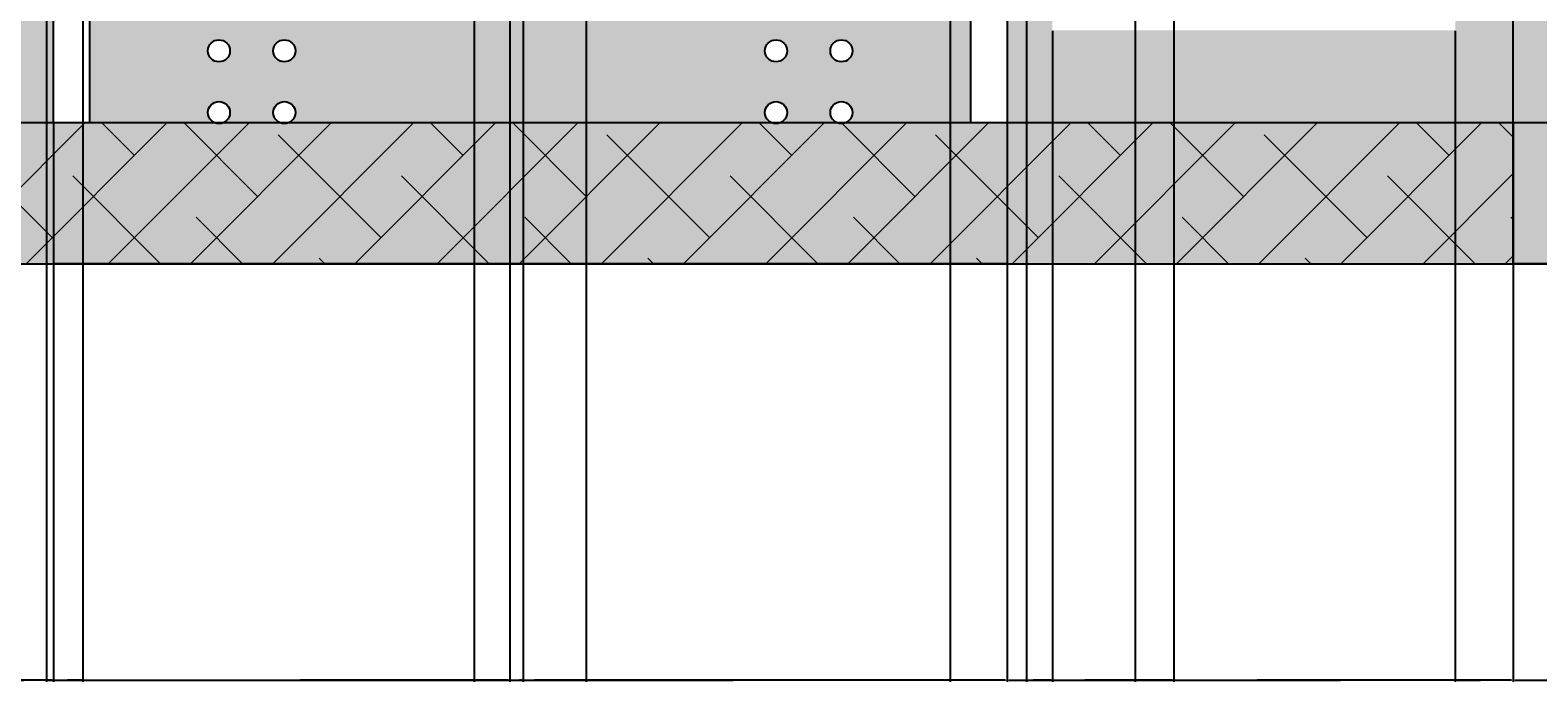
# Model space of a CAD drawing. Units: inches. Extents: x 3024 to 4744, y 1110 to 2100.
# Tile 4 of 29: x 3168 to 3332, y 1110 to 1181. Entities that reach past the tile are written whole.
import ezdxf

# ---------------------------------------------------------------- set-up
doc = ezdxf.new("R2010")
doc.units = ezdxf.units.IN
for name, color, linetype, lineweight in [('A-ANNO-DIMS', 2, 'Continuous', 18), ('A-ELEV', 7, 'Continuous', 25), ('A-ELEV-PATT', 252, 'Continuous', 13)]:
    doc.layers.add(name, color=color, linetype=linetype, lineweight=lineweight)
doc.styles.get("Standard").update_dxf_attribs({"font": 'arial.ttf'})
doc.dimstyles.get("Standard").update_dxf_attribs({"dimtxt": 0.18, "dimasz": 0.18, "dimexe": 0.18, "dimexo": 0.0625, "dimgap": 0.09, "dimtad": 0, "dimtih": 1, "dimtoh": 1, "dimdec": 1, "dimzin": 0, "dimdsep": 46, "dimlunit": 3, "dimtxsty": 'Standard', "dimcen": 0.09, "dimadec": 0, "dimazin": 0, "dimtfac": 1, "dimtdec": 1, "dimtofl": 0, "dimtmove": 0, "dimatfit": 3, "dimfxl": 1, "dimtolj": 1, "dimtzin": 0, "dimarcsym": 0})

# ---------------------------------------------------------------- blocks, each defined once
blk = doc.blocks.new('*D52')
at = {"layer": 'A-ANNO-DIMS', "color": 0, "lineweight": -2, "transparency": 16777216}
for p, q in [((3148.97, 1290.98), (3148.97, 1109.93)), ((3170.16, 1170.96), (3170.16, 1109.93)), ((3149.15, 1110.11), (3159.17, 1110.11)), ((3169.98, 1110.11), (3159.96, 1110.11))]:
    blk.add_line(p, q, dxfattribs=at)
at = {"layer": 'A-ANNO-DIMS', "color": 0, "transparency": 16777216}
for points in [[(3149.15, 1110.14), (3149.15, 1110.08), (3148.97, 1110.11)], [(3169.98, 1110.14), (3169.98, 1110.08), (3170.16, 1110.11)]]:
    blk.add_solid(points, dxfattribs=at)
at = {"layer": 'Defpoints', "color": 0, "transparency": 16777216}
for p in [(3148.97, 1291.04), (3170.16, 1171.02), (3170.16, 1110.11)]:
    blk.add_point(p, dxfattribs=at)
at = {"layer": 'A-ANNO-DIMS', "color": 0, "transparency": 16777216, "insert": (3159.57, 1110.11), "char_height": 0.18, "attachment_point": 5}
blk.add_mtext('\\A1;21.19', dxfattribs=at)
blk = doc.blocks.new('*D53')
at = {"layer": 'A-ANNO-DIMS', "color": 0, "lineweight": -2, "transparency": 16777216}
for p, q in [((3170.16, 1170.96), (3170.16, 1109.93)), ((3274.39, 1170.96), (3274.39, 1109.93)), ((3170.34, 1110.11), (3221.82, 1110.11)), ((3274.21, 1110.11), (3222.73, 1110.11))]:
    blk.add_line(p, q, dxfattribs=at)
at = {"layer": 'A-ANNO-DIMS', "color": 0, "transparency": 16777216}
for points in [[(3170.34, 1110.14), (3170.34, 1110.08), (3170.16, 1110.11)], [(3274.21, 1110.14), (3274.21, 1110.08), (3274.39, 1110.11)]]:
    blk.add_solid(points, dxfattribs=at)
at = {"layer": 'Defpoints', "color": 0, "transparency": 16777216}
for p in [(3170.16, 1171.02), (3274.39, 1171.02), (3274.39, 1110.11)]:
    blk.add_point(p, dxfattribs=at)
at = {"layer": 'A-ANNO-DIMS', "color": 0, "transparency": 16777216, "insert": (3222.27, 1110.11), "char_height": 0.18, "attachment_point": 5}
blk.add_mtext('\\A1;104.23', dxfattribs=at)
blk = doc.blocks.new('*D54')
at = {"layer": 'A-ANNO-DIMS', "color": 0, "lineweight": -2, "transparency": 16777216}
for p, q in [((3292.61, 1290.98), (3292.61, 1109.93)), ((3274.39, 1170.96), (3274.39, 1109.93)), ((3274.57, 1110.11), (3283.04, 1110.11)), ((3292.43, 1110.11), (3283.95, 1110.11))]:
    blk.add_line(p, q, dxfattribs=at)
at = {"layer": 'A-ANNO-DIMS', "color": 0, "transparency": 16777216}
for points in [[(3274.57, 1110.14), (3274.57, 1110.08), (3274.39, 1110.11)], [(3292.43, 1110.14), (3292.43, 1110.08), (3292.61, 1110.11)]]:
    blk.add_solid(points, dxfattribs=at)
at = {"layer": 'Defpoints', "color": 0, "transparency": 16777216}
for p in [(3292.61, 1291.04), (3274.39, 1171.02), (3292.61, 1110.11)]:
    blk.add_point(p, dxfattribs=at)
at = {"layer": 'A-ANNO-DIMS', "color": 0, "transparency": 16777216, "insert": (3283.5, 1110.11), "char_height": 0.18, "attachment_point": 5}
blk.add_mtext('\\A1;18.217', dxfattribs=at)
blk = doc.blocks.new('*D55')
at = {"layer": 'A-ANNO-DIMS', "color": 0, "lineweight": -2, "transparency": 16777216}
for p, q in [((3292.61, 1290.98), (3292.61, 1109.93)), ((3329.7, 1155.55), (3329.7, 1109.93)), ((3292.79, 1110.11), (3310.85, 1110.11)), ((3329.52, 1110.11), (3311.46, 1110.11))]:
    blk.add_line(p, q, dxfattribs=at)
at = {"layer": 'A-ANNO-DIMS', "color": 0, "transparency": 16777216}
for points in [[(3292.79, 1110.14), (3292.79, 1110.08), (3292.61, 1110.11)], [(3329.52, 1110.14), (3329.52, 1110.08), (3329.7, 1110.11)]]:
    blk.add_solid(points, dxfattribs=at)
at = {"layer": 'Defpoints', "color": 0, "transparency": 16777216}
for p in [(3292.61, 1291.04), (3329.7, 1155.61), (3329.7, 1110.11)]:
    blk.add_point(p, dxfattribs=at)
at = {"layer": 'A-ANNO-DIMS', "color": 0, "transparency": 16777216, "insert": (3311.15, 1110.11), "char_height": 0.18, "attachment_point": 5}
blk.add_mtext('\\A1;37.1', dxfattribs=at)
blk = doc.blocks.new('*D56')
at = {"layer": 'A-ANNO-DIMS', "color": 0, "lineweight": -2, "transparency": 16777216}
for p, q in [((3361.22, 1329.46), (3361.22, 1109.93)), ((3329.7, 1155.55), (3329.7, 1109.93)), ((3329.88, 1110.11), (3345.07, 1110.11)), ((3361.04, 1110.11), (3345.86, 1110.11))]:
    blk.add_line(p, q, dxfattribs=at)
at = {"layer": 'A-ANNO-DIMS', "color": 0, "transparency": 16777216}
for points in [[(3329.88, 1110.14), (3329.88, 1110.08), (3329.7, 1110.11)], [(3361.04, 1110.14), (3361.04, 1110.08), (3361.22, 1110.11)]]:
    blk.add_solid(points, dxfattribs=at)
at = {"layer": 'Defpoints', "color": 0, "transparency": 16777216}
for p in [(3361.22, 1329.52), (3329.7, 1155.61), (3361.22, 1110.11)]:
    blk.add_point(p, dxfattribs=at)
at = {"layer": 'A-ANNO-DIMS', "color": 0, "transparency": 16777216, "insert": (3345.46, 1110.11), "char_height": 0.18, "attachment_point": 5}
blk.add_mtext('\\A1;31.52', dxfattribs=at)
blk = doc.blocks.new('*D90')
at = {"layer": 'A-ANNO-DIMS', "color": 0, "lineweight": -2, "transparency": 16777216}
for p, q in [((3173.4, 1798.98), (3173.4, 1109.93)), ((3169.4, 1794.98), (3169.4, 1109.93)), ((3169.58, 1110.11), (3171.07, 1110.11)), ((3173.22, 1110.11), (3171.72, 1110.11))]:
    blk.add_line(p, q, dxfattribs=at)
at = {"layer": 'A-ANNO-DIMS', "color": 0, "transparency": 16777216}
for points in [[(3169.58, 1110.14), (3169.58, 1110.08), (3169.4, 1110.11)], [(3173.22, 1110.14), (3173.22, 1110.08), (3173.4, 1110.11)]]:
    blk.add_solid(points, dxfattribs=at)
at = {"layer": 'Defpoints', "color": 0, "transparency": 16777216}
for p in [(3173.4, 1799.04), (3169.4, 1795.04), (3173.4, 1110.11)]:
    blk.add_point(p, dxfattribs=at)
at = {"layer": 'A-ANNO-DIMS', "color": 0, "transparency": 16777216, "insert": (3171.4, 1110.11), "char_height": 0.18, "attachment_point": 5}
blk.add_mtext('\\A1;4.00', dxfattribs=at)
blk = doc.blocks.new('*D91')
at = {"layer": 'A-ANNO-DIMS', "color": 0, "lineweight": -2, "transparency": 16777216}
for p, q in [((3173.4, 1798.98), (3173.4, 1109.93)), ((3220.05, 1798.98), (3220.05, 1109.93)), ((3173.58, 1110.11), (3196.33, 1110.11)), ((3219.87, 1110.11), (3197.12, 1110.11))]:
    blk.add_line(p, q, dxfattribs=at)
at = {"layer": 'A-ANNO-DIMS', "color": 0, "transparency": 16777216}
for points in [[(3173.58, 1110.14), (3173.58, 1110.08), (3173.4, 1110.11)], [(3219.87, 1110.14), (3219.87, 1110.08), (3220.05, 1110.11)]]:
    blk.add_solid(points, dxfattribs=at)
at = {"layer": 'Defpoints', "color": 0, "transparency": 16777216}
for p in [(3173.4, 1799.04), (3220.05, 1799.04), (3220.05, 1110.11)]:
    blk.add_point(p, dxfattribs=at)
at = {"layer": 'A-ANNO-DIMS', "color": 0, "transparency": 16777216, "insert": (3196.72, 1110.11), "char_height": 0.18, "attachment_point": 5}
blk.add_mtext('\\A1;46.65', dxfattribs=at)
blk = doc.blocks.new('*D92')
at = {"layer": 'A-ANNO-DIMS', "color": 0, "lineweight": -2, "transparency": 16777216}
for p, q in [((3220.05, 1798.98), (3220.05, 1109.93)), ((3221.52, 1798.98), (3221.52, 1109.93)), ((3220.23, 1110.11), (3220.47, 1110.11)), ((3221.34, 1110.11), (3221.1, 1110.11))]:
    blk.add_line(p, q, dxfattribs=at)
at = {"layer": 'A-ANNO-DIMS', "color": 0, "transparency": 16777216}
for points in [[(3220.23, 1110.14), (3220.23, 1110.08), (3220.05, 1110.11)], [(3221.34, 1110.14), (3221.34, 1110.08), (3221.52, 1110.11)]]:
    blk.add_solid(points, dxfattribs=at)
at = {"layer": 'Defpoints', "color": 0, "transparency": 16777216}
for p in [(3220.05, 1799.04), (3221.52, 1799.04), (3221.52, 1110.11)]:
    blk.add_point(p, dxfattribs=at)
at = {"layer": 'A-ANNO-DIMS', "color": 0, "transparency": 16777216, "insert": (3220.79, 1110.11), "char_height": 0.18, "attachment_point": 5}
blk.add_mtext('\\A1;1.47', dxfattribs=at)
blk = doc.blocks.new('*D93')
at = {"layer": 'A-ANNO-DIMS', "color": 0, "lineweight": -2, "transparency": 16777216}
for p, q in [((3221.52, 1798.98), (3221.52, 1109.93)), ((3268.18, 1798.98), (3268.18, 1109.93)), ((3221.7, 1110.11), (3244.45, 1110.11)), ((3268, 1110.11), (3245.25, 1110.11))]:
    blk.add_line(p, q, dxfattribs=at)
at = {"layer": 'A-ANNO-DIMS', "color": 0, "transparency": 16777216}
for points in [[(3221.7, 1110.14), (3221.7, 1110.08), (3221.52, 1110.11)], [(3268, 1110.14), (3268, 1110.08), (3268.18, 1110.11)]]:
    blk.add_solid(points, dxfattribs=at)
at = {"layer": 'Defpoints', "color": 0, "transparency": 16777216}
for p in [(3221.52, 1799.04), (3268.18, 1799.04), (3268.18, 1110.11)]:
    blk.add_point(p, dxfattribs=at)
at = {"layer": 'A-ANNO-DIMS', "color": 0, "transparency": 16777216, "insert": (3244.85, 1110.11), "char_height": 0.18, "attachment_point": 5}
blk.add_mtext('\\A1;46.65', dxfattribs=at)
blk = doc.blocks.new('*D94')
at = {"layer": 'A-ANNO-DIMS', "color": 0, "lineweight": -2, "transparency": 16777216}
for p, q in [((3276.51, 1794.98), (3276.51, 1109.93)), ((3288.38, 1794.98), (3288.38, 1109.93)), ((3276.69, 1110.11), (3281.99, 1110.11)), ((3288.2, 1110.11), (3282.9, 1110.11))]:
    blk.add_line(p, q, dxfattribs=at)
at = {"layer": 'A-ANNO-DIMS', "color": 0, "transparency": 16777216}
for points in [[(3276.69, 1110.14), (3276.69, 1110.08), (3276.51, 1110.11)], [(3288.2, 1110.14), (3288.2, 1110.08), (3288.38, 1110.11)]]:
    blk.add_solid(points, dxfattribs=at)
at = {"layer": 'Defpoints', "color": 0, "transparency": 16777216}
for p in [(3276.51, 1795.04), (3288.38, 1795.04), (3288.38, 1110.11)]:
    blk.add_point(p, dxfattribs=at)
at = {"layer": 'A-ANNO-DIMS', "color": 0, "transparency": 16777216, "insert": (3282.44, 1110.11), "char_height": 0.18, "attachment_point": 5}
blk.add_mtext('\\A1;11.866', dxfattribs=at)
blk = doc.blocks.new('*D105')
at = {"layer": 'A-ANNO-DIMS', "color": 0, "lineweight": -2, "transparency": 16777216}
for p, q in [((3164.38, 1181.06), (3164.38, 1109.93)), ((3170.16, 1170.96), (3170.16, 1109.93)), ((3164.56, 1110.11), (3166.95, 1110.11)), ((3169.98, 1110.11), (3167.59, 1110.11))]:
    blk.add_line(p, q, dxfattribs=at)
at = {"layer": 'A-ANNO-DIMS', "color": 0, "transparency": 16777216}
for points in [[(3164.56, 1110.14), (3164.56, 1110.08), (3164.38, 1110.11)], [(3169.98, 1110.14), (3169.98, 1110.08), (3170.16, 1110.11)]]:
    blk.add_solid(points, dxfattribs=at)
at = {"layer": 'Defpoints', "color": 0, "transparency": 16777216}
for p in [(3164.38, 1181.12), (3170.16, 1171.02), (3170.16, 1110.11)]:
    blk.add_point(p, dxfattribs=at)
at = {"layer": 'A-ANNO-DIMS', "color": 0, "transparency": 16777216, "insert": (3167.27, 1110.11), "char_height": 0.18, "attachment_point": 5}
blk.add_mtext('\\A1;5.78', dxfattribs=at)
blk = doc.blocks.new('*D109')
at = {"layer": 'A-ANNO-DIMS', "color": 0, "lineweight": -2, "transparency": 16777216}
for p, q in [((3216.16, 1185.89), (3216.16, 1109.93)), ((3228.39, 1185.89), (3228.39, 1109.93)), ((3216.34, 1110.11), (3221.82, 1110.11)), ((3228.21, 1110.11), (3222.73, 1110.11))]:
    blk.add_line(p, q, dxfattribs=at)
at = {"layer": 'A-ANNO-DIMS', "color": 0, "transparency": 16777216}
for points in [[(3216.34, 1110.14), (3216.34, 1110.08), (3216.16, 1110.11)], [(3228.21, 1110.14), (3228.21, 1110.08), (3228.39, 1110.11)]]:
    blk.add_solid(points, dxfattribs=at)
at = {"layer": 'Defpoints', "color": 0, "transparency": 16777216}
for p in [(3216.16, 1185.95), (3228.39, 1185.95), (3228.39, 1110.11)]:
    blk.add_point(p, dxfattribs=at)
at = {"layer": 'A-ANNO-DIMS', "color": 0, "transparency": 16777216, "insert": (3222.27, 1110.11), "char_height": 0.18, "attachment_point": 5}
blk.add_mtext('\\A1;12.223', dxfattribs=at)
blk = doc.blocks.new('*D110')
at = {"layer": 'A-ANNO-DIMS', "color": 0, "lineweight": -2, "transparency": 16777216}
for p, q in [((3279.36, 1181.06), (3279.36, 1109.93)), ((3274.39, 1170.96), (3274.39, 1109.93)), ((3274.57, 1110.11), (3276.49, 1110.11)), ((3279.18, 1110.11), (3277.25, 1110.11))]:
    blk.add_line(p, q, dxfattribs=at)
at = {"layer": 'A-ANNO-DIMS', "color": 0, "transparency": 16777216}
for points in [[(3274.57, 1110.14), (3274.57, 1110.08), (3274.39, 1110.11)], [(3279.18, 1110.14), (3279.18, 1110.08), (3279.36, 1110.11)]]:
    blk.add_solid(points, dxfattribs=at)
at = {"layer": 'Defpoints', "color": 0, "transparency": 16777216}
for p in [(3279.36, 1181.12), (3274.39, 1171.02), (3279.36, 1110.11)]:
    blk.add_point(p, dxfattribs=at)
at = {"layer": 'A-ANNO-DIMS', "color": 0, "transparency": 16777216, "insert": (3276.87, 1110.11), "char_height": 0.18, "attachment_point": 5}
blk.add_mtext('\\A1;4.971', dxfattribs=at)
blk = doc.blocks.new('*D111')
at = {"layer": 'A-ANNO-DIMS', "color": 0, "lineweight": -2, "transparency": 16777216}
for p, q in [((3279.36, 1181.06), (3279.36, 1109.93)), ((3323.37, 1181.06), (3323.37, 1109.93)), ((3279.54, 1110.11), (3300.98, 1110.11)), ((3323.19, 1110.11), (3301.74, 1110.11))]:
    blk.add_line(p, q, dxfattribs=at)
at = {"layer": 'A-ANNO-DIMS', "color": 0, "transparency": 16777216}
for points in [[(3279.54, 1110.14), (3279.54, 1110.08), (3279.36, 1110.11)], [(3323.19, 1110.14), (3323.19, 1110.08), (3323.37, 1110.11)]]:
    blk.add_solid(points, dxfattribs=at)
at = {"layer": 'Defpoints', "color": 0, "transparency": 16777216}
for p in [(3279.36, 1181.12), (3323.37, 1181.12), (3323.37, 1110.11)]:
    blk.add_point(p, dxfattribs=at)
at = {"layer": 'A-ANNO-DIMS', "color": 0, "transparency": 16777216, "insert": (3301.36, 1110.11), "char_height": 0.18, "attachment_point": 5}
blk.add_mtext('\\A1;44.01', dxfattribs=at)
blk = doc.blocks.new('*D112')
at = {"layer": 'A-ANNO-DIMS', "color": 0, "lineweight": -2, "transparency": 16777216}
for p, q in [((3323.37, 1181.06), (3323.37, 1109.93)), ((3329.7, 1170.96), (3329.7, 1109.93)), ((3323.55, 1110.11), (3326.14, 1110.11)), ((3329.52, 1110.11), (3326.93, 1110.11))]:
    blk.add_line(p, q, dxfattribs=at)
at = {"layer": 'A-ANNO-DIMS', "color": 0, "transparency": 16777216}
for points in [[(3323.55, 1110.14), (3323.55, 1110.08), (3323.37, 1110.11)], [(3329.52, 1110.14), (3329.52, 1110.08), (3329.7, 1110.11)]]:
    blk.add_solid(points, dxfattribs=at)
at = {"layer": 'Defpoints', "color": 0, "transparency": 16777216}
for p in [(3323.37, 1181.12), (3329.7, 1171.02), (3329.7, 1110.11)]:
    blk.add_point(p, dxfattribs=at)
at = {"layer": 'A-ANNO-DIMS', "color": 0, "transparency": 16777216, "insert": (3326.54, 1110.11), "char_height": 0.18, "attachment_point": 5}
blk.add_mtext('\\A1;6.334', dxfattribs=at)
blk = doc.blocks.new('*D120')
at = {"layer": 'A-ANNO-DIMS', "color": 0, "lineweight": -2, "transparency": 16777216}
for p, q in [((3270.45, 1271.61), (3786.83, 1271.61)), ((3786.65, 1271.43), (3786.65, 1221.5)), ((3786.65, 1171.2), (3786.65, 1221.14)), ((3274.45, 1171.02), (3786.83, 1171.02))]:
    blk.add_line(p, q, dxfattribs=at)
at = {"layer": 'A-ANNO-DIMS', "color": 0, "transparency": 16777216}
for points in [[(3786.62, 1271.43), (3786.68, 1271.43), (3786.65, 1271.61)], [(3786.62, 1171.2), (3786.68, 1171.2), (3786.65, 1171.02)]]:
    blk.add_solid(points, dxfattribs=at)
at = {"layer": 'Defpoints', "color": 0, "transparency": 16777216}
for p in [(3270.39, 1271.61), (3786.65, 1271.61), (3274.39, 1171.02)]:
    blk.add_point(p, dxfattribs=at)
at = {"layer": 'A-ANNO-DIMS', "color": 0, "transparency": 16777216, "insert": (3786.65, 1221.32), "char_height": 0.18, "attachment_point": 5}
blk.add_mtext('\\A1;100.59', dxfattribs=at)
blk = doc.blocks.new('*D122')
at = {"layer": 'A-ANNO-DIMS', "color": 0, "lineweight": -2, "transparency": 16777216}
for p, q in [((3228.45, 1185.95), (3786.83, 1185.95)), ((3786.65, 1185.77), (3786.65, 1178.67)), ((3786.65, 1171.2), (3786.65, 1178.31)), ((3270.45, 1171.02), (3786.83, 1171.02))]:
    blk.add_line(p, q, dxfattribs=at)
at = {"layer": 'A-ANNO-DIMS', "color": 0, "transparency": 16777216}
for points in [[(3786.62, 1185.77), (3786.68, 1185.77), (3786.65, 1185.95)], [(3786.62, 1171.2), (3786.68, 1171.2), (3786.65, 1171.02)]]:
    blk.add_solid(points, dxfattribs=at)
at = {"layer": 'Defpoints', "color": 0, "transparency": 16777216}
for p in [(3228.39, 1185.95), (3270.39, 1171.02), (3786.65, 1171.02)]:
    blk.add_point(p, dxfattribs=at)
at = {"layer": 'A-ANNO-DIMS', "color": 0, "transparency": 16777216, "insert": (3786.65, 1178.49), "char_height": 0.18, "attachment_point": 5}
blk.add_mtext('\\A1;14.928', dxfattribs=at)

msp = doc.modelspace()

# ---------------------------------------------------------------- hatches: boundary and pattern name
at = {"layer": 'A-ELEV-PATT'}
h = msp.add_hatch(color=256, dxfattribs=at)
h.dxf.hatch_style = 1
h.paths.add_polyline_path([(3335.1044, 2043.5286), (3329.7033, 2043.5286), (3329.7033, 1155.6112), (3335.1044, 1155.6112)])
h.paths.add_polyline_path([(3481.2411, 2043.5286), (3335.1044, 2043.5286), (3335.1044, 1155.6112), (3481.2411, 1155.6112)])
h.paths.add_polyline_path([(3449.7202, 1329.5246), (3361.2242, 1329.5246), (3361.2242, 1436.6064), (3449.7202, 1436.6064)], flags=16)
h.paths.add_polyline_path([(3445.7202, 1333.5246), (3365.2242, 1333.5246), (3365.2242, 1432.6064), (3445.7202, 1432.6064)], flags=0)
h.paths.add_polyline_path([(3449.7202, 1455.5246), (3361.2242, 1455.5246), (3361.2242, 1562.6064), (3449.7202, 1562.6064)], flags=16)
h.paths.add_polyline_path([(3445.7202, 1459.5246), (3365.2242, 1459.5246), (3365.2242, 1558.6064), (3445.7202, 1558.6064)], flags=0)
h.paths.add_polyline_path([(3449.7202, 1581.5246), (3361.2242, 1581.5246), (3361.2242, 1688.6064), (3449.7202, 1688.6064)], flags=16)
h.paths.add_polyline_path([(3445.7202, 1585.5246), (3365.2242, 1585.5246), (3365.2242, 1684.6064), (3445.7202, 1684.6064)], flags=0)
h.paths.add_polyline_path([(3449.7202, 1707.5246), (3361.2242, 1707.5246), (3361.2242, 1814.6064), (3449.7202, 1814.6064)], flags=16)
h.paths.add_polyline_path([(3445.7202, 1711.5246), (3365.2242, 1711.5246), (3365.2242, 1810.6064), (3445.7202, 1810.6064)], flags=0)
h.paths.add_polyline_path([(3449.7202, 1833.5246), (3361.2242, 1833.5246), (3361.2242, 1940.6064), (3449.7202, 1940.6064)], flags=16)
h.paths.add_polyline_path([(3445.7202, 1837.5246), (3365.2242, 1837.5246), (3365.2242, 1936.6064), (3445.7202, 1936.6064)], flags=0)
h = msp.add_hatch(color=256, dxfattribs=at)
h.dxf.hatch_style = 1
h.paths.add_polyline_path([(3329.7033, 1275.6112), (3274.3877, 1275.6112), (3274.3877, 1171.0239), (3329.7033, 1171.0239)])
h.paths.add_polyline_path([(3323.3693, 1246.0161), (3279.3583, 1246.0161), (3279.3583, 1270.5642), (3323.3693, 1270.5642)], flags=16)
h.paths.add_polyline_path([(3323.3693, 1238.118), (3323.3693, 1213.5699), (3279.3583, 1213.5699), (3279.3583, 1238.118)], flags=16)
h.paths.add_polyline_path([(3323.3693, 1205.6718), (3323.3693, 1181.1236), (3279.3583, 1181.1236), (3279.3583, 1205.6718)], flags=16)
h.paths.add_polyline_path([(3170.1608, 1275.6112), (3112.3838, 1275.6112), (3112.3838, 1171.0239), (3118.1176, 1171.0239), (3170.1608, 1171.0239)])
h.paths.add_polyline_path([(3120.3696, 1246.0161), (3120.3696, 1270.5642), (3164.3806, 1270.5642), (3164.3806, 1246.0161)], flags=16)
h.paths.add_polyline_path([(3120.3696, 1238.118), (3164.3806, 1238.118), (3164.3806, 1213.5699), (3120.3696, 1213.5699)], flags=16)
h.paths.add_polyline_path([(3120.3696, 1205.6718), (3164.3806, 1205.6718), (3164.3806, 1181.1236), (3120.3696, 1181.1236)], flags=16)
h = msp.add_hatch(color=256, dxfattribs=at)
h.dxf.hatch_style = 1
h.paths.add_polyline_path([(3270.3877, 1271.6112), (3174.1608, 1271.6112), (3174.1608, 1171.0239), (3187.7692, 1171.0239, -0.29659686), (3187.0515, 1172.1274, -1), (3189.4658, 1172.1274, -0.29659686), (3188.7481, 1171.0239), (3194.9159, 1171.0239, -0.29659686), (3194.1982, 1172.1274, -1), (3196.6124, 1172.1274, -0.29659686), (3195.8947, 1171.0239), (3248.6539, 1171.0239, -0.29659686), (3247.9362, 1172.1274, -1), (3250.3504, 1172.1274, -0.29659686), (3249.6327, 1171.0239), (3255.8005, 1171.0239, -0.29659686), (3255.0828, 1172.1274, -1), (3257.4971, 1172.1274, -0.29659686), (3256.7794, 1171.0239), (3270.3877, 1171.0239)])
h.paths.add_polyline_path([(3196.6124, 1256.2276, -1), (3194.1982, 1256.2276, -1)], flags=16)
h.paths.add_polyline_path([(3196.6124, 1249.4899, -1), (3194.1982, 1249.4899, -1)], flags=16)
h.paths.add_polyline_path([(3216.163, 1245.2708), (3228.3856, 1245.2708), (3228.3856, 1185.9515), (3216.163, 1185.9515)], flags=16)
h.paths.add_polyline_path([(3187.0515, 1256.2276, -1), (3189.4658, 1256.2276, -1)], flags=16)
h.paths.add_polyline_path([(3189.4658, 1249.4899, -1), (3187.0515, 1249.4899, -1)], flags=16)
h.paths.add_polyline_path([(3196.6124, 1236.8869, -1), (3194.1982, 1236.8869, -1)], flags=16)
h.paths.add_polyline_path([(3189.4658, 1236.8869, -1), (3187.0515, 1236.8869, -1)], flags=16)
h.paths.add_polyline_path([(3196.6124, 1230.1493, -1), (3194.1982, 1230.1493, -1)], flags=16)
h.paths.add_polyline_path([(3189.4658, 1230.1493, -1), (3187.0515, 1230.1493, -1)], flags=16)
h.paths.add_polyline_path([(3250.3504, 1256.2276, -1), (3247.9362, 1256.2276, -1)], flags=16)
h.paths.add_polyline_path([(3250.3504, 1249.4899, -1), (3247.9362, 1249.4899, -1)], flags=16)
h.paths.add_polyline_path([(3196.6124, 1217.5463, -1), (3194.1982, 1217.5463, -1)], flags=16)
h.paths.add_polyline_path([(3250.3504, 1236.8869, -1), (3247.9362, 1236.8869, -1)], flags=16)
h.paths.add_polyline_path([(3189.4658, 1217.5463, -1), (3187.0515, 1217.5463, -1)], flags=16)
h.paths.add_polyline_path([(3257.4971, 1256.2276, -1), (3255.0828, 1256.2276, -1)], flags=16)
h.paths.add_polyline_path([(3257.4971, 1249.4899, -1), (3255.0828, 1249.4899, -1)], flags=16)
h.paths.add_polyline_path([(3250.3504, 1230.1493, -1), (3247.9362, 1230.1493, -1)], flags=16)
h.paths.add_polyline_path([(3196.6124, 1210.8086, -1), (3194.1982, 1210.8086, -1)], flags=16)
h.paths.add_polyline_path([(3189.4658, 1210.8086, -1), (3187.0515, 1210.8086, -1)], flags=16)
h.paths.add_polyline_path([(3257.4971, 1236.8869, -1), (3255.0828, 1236.8869, -1)], flags=16)
h.paths.add_polyline_path([(3257.4971, 1230.1493, -1), (3255.0828, 1230.1493, -1)], flags=16)
h.paths.add_polyline_path([(3250.3504, 1217.5463, -1), (3247.9362, 1217.5463, -1)], flags=16)
h.paths.add_polyline_path([(3196.6124, 1198.2057, -1), (3194.1982, 1198.2057, -1)], flags=16)
h.paths.add_polyline_path([(3250.3504, 1210.8086, -1), (3247.9362, 1210.8086, -1)], flags=16)
h.paths.add_polyline_path([(3257.4971, 1217.5463, -1), (3255.0828, 1217.5463, -1)], flags=16)
h.paths.add_polyline_path([(3189.4658, 1198.2057, -1), (3187.0515, 1198.2057, -1)], flags=16)
h.paths.add_polyline_path([(3257.4971, 1210.8086, -1), (3255.0828, 1210.8086, -1)], flags=16)
h.paths.add_polyline_path([(3196.6124, 1191.468, -1), (3194.1982, 1191.468, -1)], flags=16)
h.paths.add_polyline_path([(3189.4658, 1191.468, -1), (3187.0515, 1191.468, -1)], flags=16)
h.paths.add_polyline_path([(3250.3504, 1198.2057, -1), (3247.9362, 1198.2057, -1)], flags=16)
h.paths.add_polyline_path([(3257.4971, 1198.2057, -1), (3255.0828, 1198.2057, -1)], flags=16)
h.paths.add_polyline_path([(3250.3504, 1191.468, -1), (3247.9362, 1191.468, -1)], flags=16)
h.paths.add_polyline_path([(3196.6124, 1178.8651, -1), (3194.1982, 1178.8651, -1)], flags=16)
h.paths.add_polyline_path([(3257.4971, 1191.468, -1), (3255.0828, 1191.468, -1)], flags=16)
h.paths.add_polyline_path([(3189.4658, 1178.8651, -1), (3187.0515, 1178.8651, -1)], flags=16)
h.paths.add_polyline_path([(3250.3504, 1178.8651, -1), (3247.9362, 1178.8651, -1)], flags=16)
h.paths.add_polyline_path([(3257.4971, 1178.8651, -1), (3255.0828, 1178.8651, -1)], flags=16)
h = msp.add_hatch(color=256, dxfattribs=at)
h.dxf.hatch_style = 1
h.paths.add_polyline_path([(3329.7033, 1171.0239), (3256.7794, 1171.0239, -0.21182003), (3255.8005, 1171.0239), (3249.6327, 1171.0239, -0.21182003), (3248.6539, 1171.0239), (3195.8947, 1171.0239, -0.21182003), (3194.9159, 1171.0239), (3188.7481, 1171.0239, -0.21182003), (3187.7692, 1171.0239), (3118.1176, 1171.0239), (3115.5754, 1168.0828), (3115.5754, 1155.6112), (3329.7033, 1155.6112)])
h.paths.add_polyline_path([(3101.9647, 1168.0828), (3103.2358, 1169.5534), (3069.7937, 1169.5534), (3069.7937, 1155.6112), (3101.9647, 1155.6112)])
h.paths.add_polyline_path([(3115.5754, 1168.0828), (3101.9647, 1168.0828), (3101.9647, 1155.6112), (3105.4722, 1155.6112), (3115.5754, 1155.6112)])
h.paths.add_polyline_path([(3118.1176, 1171.0239), (3104.5069, 1171.0239), (3101.9647, 1168.0828), (3115.5754, 1168.0828)])
h.paths.add_polyline_path([(3105.4722, 1265.3254), (3075.5369, 1241.4341), (3075.5369, 1169.5534), (3103.2358, 1169.5534), (3104.5069, 1171.0239), (3105.4722, 1171.0239)])
h.paths.add_polyline_path([(3105.4722, 1265.3254), (3105.4722, 1269.9091), (3069.7937, 1241.4341), (3075.5369, 1241.4341)])
h.paths.add_polyline_path([(3075.5369, 1241.4341), (3069.7937, 1241.4341), (3069.7937, 1169.5534), (3075.5369, 1169.5534)])
h.paths.add_polyline_path([(3735.4075, 1241.4341), (3705.4722, 1265.3254), (3705.4722, 1169.5534), (3735.4075, 1169.5534)])
h.paths.add_polyline_path([(3705.4722, 1269.9091), (3705.4722, 1265.3254), (3735.4075, 1241.4341), (3741.1507, 1241.4341)])
h.paths.add_polyline_path([(3741.1507, 1241.4341), (3735.4075, 1241.4341), (3735.4075, 1169.5534), (3741.1507, 1169.5534)])
h.paths.add_polyline_path([(3741.1507, 1169.5534), (3735.4075, 1169.5534), (3705.4722, 1169.5534), (3705.4722, 1155.6112), (3741.1507, 1155.6112)])
h = msp.add_hatch(dxfattribs=at)
h.set_pattern_fill('ANSI38', color=256, scale=2)
h.paths.add_polyline_path([(3101.9647, 1168.0828), (3103.2358, 1169.5534), (3069.7937, 1169.5534), (3069.7937, 1155.6112), (3101.9647, 1155.6112)])
h.paths.add_polyline_path([(3115.5754, 1168.0828), (3101.9647, 1168.0828), (3101.9647, 1155.6112), (3105.4722, 1155.6112), (3115.5754, 1155.6112)])
h.paths.add_polyline_path([(3118.1176, 1171.0239), (3104.5069, 1171.0239), (3101.9647, 1168.0828), (3115.5754, 1168.0828)])
h.paths.add_polyline_path([(3329.7033, 1171.0239), (3256.7794, 1171.0239, -0.21182003), (3255.8005, 1171.0239), (3249.6327, 1171.0239, -0.21182003), (3248.6539, 1171.0239), (3195.8947, 1171.0239, -0.21182003), (3194.9159, 1171.0239), (3188.7481, 1171.0239, -0.21182003), (3187.7692, 1171.0239), (3118.1176, 1171.0239), (3115.5754, 1168.0828), (3115.5754, 1155.6112), (3329.7033, 1155.6112)])
h.paths.add_polyline_path([(3741.1507, 1169.5534), (3735.4075, 1169.5534), (3705.4722, 1169.5534), (3705.4722, 1155.6112), (3741.1507, 1155.6112)])

# ---------------------------------------------------------------- linework, layer by layer
at = {"layer": 'A-ELEV'}
for p, q in [((3118.1176, 1171.0239), (3329.7033, 1171.0239)), ((3118.1176, 1171.0239), (3329.7033, 1171.0239)), ((3105.4722, 1155.6112), (3705.4722, 1155.6112)), ((3105.4722, 1155.6112), (3705.4722, 1155.6112))]:
    msp.add_line(p, q, dxfattribs=at)
for points in [[(3481.2411, 1155.6112), (3329.7033, 1155.6112), (3329.7033, 2043.5286), (3481.2411, 2043.5286)], [(3329.7033, 2043.5286), (3335.1044, 2043.5286), (3335.1044, 1155.6112), (3329.7033, 1155.6112)], [(3481.2411, 1155.6112), (3329.7033, 1155.6112), (3329.7033, 2043.5286), (3481.2411, 2043.5286)], [(3329.7033, 2043.5286), (3335.1044, 2043.5286), (3335.1044, 1155.6112), (3329.7033, 1155.6112)]]:
    msp.add_lwpolyline(points, close=True, dxfattribs=at)
for points in [[(3170.1608, 1171.0239), (3170.1608, 1275.6112), (3274.3877, 1275.6112), (3274.3877, 1171.0239)], [(3170.1608, 1171.0239), (3170.1608, 1275.6112), (3274.3877, 1275.6112), (3274.3877, 1171.0239)], [(3174.1608, 1171.0239), (3174.1608, 1271.6112), (3270.3877, 1271.6112), (3270.3877, 1171.0239)], [(3174.1608, 1171.0239), (3174.1608, 1271.6112), (3270.3877, 1271.6112), (3270.3877, 1171.0239)], [(3274.3877, 1155.6112), (3170.1608, 1155.6112)]]:
    msp.add_lwpolyline(points, dxfattribs=at)
for centre in [(3188.2586, 1178.8651), (3188.2586, 1178.8651), (3195.4053, 1178.8651), (3195.4053, 1178.8651), (3249.1433, 1178.8651), (3249.1433, 1178.8651), (3256.2899, 1178.8651), (3256.2899, 1178.8651), (3188.2586, 1172.1274), (3188.2586, 1172.1274), (3195.4053, 1172.1274), (3195.4053, 1172.1274), (3249.1433, 1172.1274), (3249.1433, 1172.1274), (3256.2899, 1172.1274), (3256.2899, 1172.1274)]:
    msp.add_circle(centre, 1.2071, dxfattribs=at)

# ---------------------------------------------------------------- dimensions: what is measured, and where the dimension line sits
at = {"layer": 'A-ANNO-DIMS'}
for base, p1, p2, override, picture, middle in [((3173.3964, 1110.1112), (3169.3964, 1795.0431), (3173.3964, 1799.0431), {"dimdec": 2, "dimlfac": 1, "dimrnd": 0, "dimzin": 0, "dimdsep": 46, "dimlunit": 2}, '*D90', (3171.3964, 1110.1112)), ((3220.0505, 1110.1112), (3173.3964, 1799.0431), (3220.0505, 1799.0431), {"dimdec": 2, "dimlfac": 1, "dimrnd": 0, "dimzin": 0, "dimdsep": 46, "dimlunit": 2}, '*D91', (3196.7234, 1110.1112)), ((3221.5241, 1110.1112), (3220.0505, 1799.0431), (3221.5241, 1799.0431), {"dimdec": 2, "dimlfac": 1, "dimrnd": 0, "dimzin": 0, "dimdsep": 46, "dimlunit": 2}, '*D92', (3220.7873, 1110.1112)), ((3268.1781, 1110.1112), (3221.5241, 1799.0431), (3268.1781, 1799.0431), {"dimdec": 2, "dimlfac": 1, "dimrnd": 0, "dimzin": 0, "dimdsep": 46, "dimlunit": 2}, '*D93', (3244.8511, 1110.1112)), ((3288.37586, 1110.111173), (3276.509363, 1795.043127), (3288.37586, 1795.043127), {"dimdec": 3, "dimlfac": 1, "dimrnd": 0, "dimzin": 0, "dimdsep": 46, "dimlunit": 2}, '*D94', (3282.442612, 1110.111173)), ((3361.2242, 1110.1112), (3329.7033, 1155.6112), (3361.2242, 1329.5246), {"dimdec": 2, "dimlfac": 1, "dimrnd": 0, "dimzin": 0, "dimdsep": 46, "dimlunit": 2}, '*D56', (3345.4638, 1110.1112)), ((3170.1608, 1110.1112), (3148.9694, 1291.0431), (3170.1608, 1171.0239), {"dimdec": 2, "dimlfac": 1, "dimrnd": 0, "dimzin": 0, "dimdsep": 46, "dimlunit": 2}, '*D52', (3159.5651, 1110.1112)), ((3292.6051, 1110.1112), (3274.3877, 1171.0239), (3292.6051, 1291.0431), {"dimdec": 3, "dimlfac": 1, "dimrnd": 0, "dimzin": 0, "dimdsep": 46, "dimlunit": 2}, '*D54', (3283.4964, 1110.1112)), ((3329.7033, 1110.1112), (3292.6051, 1291.0431), (3329.7033, 1155.6112), {"dimdec": 1, "dimlfac": 1, "dimrnd": 0, "dimzin": 0, "dimdsep": 46, "dimlunit": 2}, '*D55', (3311.1542, 1110.1112)), ((3228.3856, 1110.1112), (3216.163, 1185.9515), (3228.3856, 1185.9515), {"dimdec": 3, "dimlfac": 1, "dimrnd": 0, "dimzin": 0, "dimdsep": 46, "dimlunit": 2}, '*D109', (3222.2743, 1110.1112)), ((3170.1608, 1110.1112), (3164.3806, 1181.1236), (3170.1608, 1171.0239), {"dimdec": 2, "dimlfac": 1, "dimrnd": 0, "dimzin": 0, "dimdsep": 46, "dimlunit": 2}, '*D105', (3167.2707, 1110.1112)), ((3279.3583, 1110.1112), (3274.3877, 1171.0239), (3279.3583, 1181.1236), {"dimdec": 3, "dimlfac": 1, "dimrnd": 0, "dimzin": 0, "dimdsep": 46, "dimlunit": 2}, '*D110', (3276.873, 1110.1112)), ((3323.3693, 1110.1112), (3279.3583, 1181.1236), (3323.3693, 1181.1236), {"dimdec": 2, "dimlfac": 1, "dimrnd": 0, "dimzin": 0, "dimdsep": 46, "dimlunit": 2}, '*D111', (3301.3638, 1110.1112)), ((3329.7033, 1110.1112), (3323.3693, 1181.1236), (3329.7033, 1171.0239), {"dimdec": 3, "dimlfac": 1, "dimrnd": 0, "dimzin": 0, "dimdsep": 46, "dimlunit": 2}, '*D112', (3326.5363, 1110.1112)), ((3274.3877, 1110.1112), (3170.1608, 1171.0239), (3274.3877, 1171.0239), {"dimdec": 2, "dimlfac": 1, "dimrnd": 0, "dimzin": 0, "dimdsep": 46, "dimlunit": 2}, '*D53', (3222.2743, 1110.1112))]:
    dim = msp.add_linear_dim(base=base, p1=p1, p2=p2, dimstyle='Standard', override=override, dxfattribs=at)
    dim.commit()
    dim.dimension.update_dxf_attribs({"geometry": picture, "text_midpoint": middle})
for base, p1, p2, override, picture, middle in [((3786.6507, 1271.6112), (3274.3877, 1171.0239), (3270.3877, 1271.6112), {"dimdec": 2, "dimlfac": 1, "dimrnd": 0, "dimzin": 0, "dimdsep": 46, "dimlunit": 2}, '*D120', (3786.6507, 1221.3176)), ((3786.6507, 1171.0239), (3228.3856, 1185.9515), (3270.3877, 1171.0239), {"dimdec": 3, "dimlfac": 1, "dimrnd": 0, "dimzin": 0, "dimdsep": 46, "dimlunit": 2}, '*D122', (3786.6507, 1178.4877))]:
    dim = msp.add_linear_dim(base=base, p1=p1, p2=p2, angle=90, dimstyle='Standard', override=override, dxfattribs=at)
    dim.commit()
    dim.dimension.update_dxf_attribs({"geometry": picture, "text_midpoint": middle})

doc.saveas('drawing.dxf')
